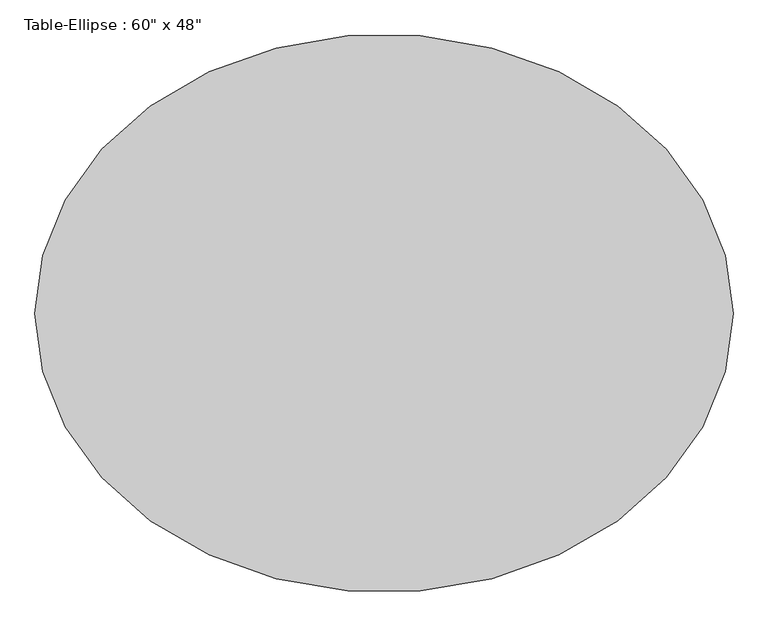
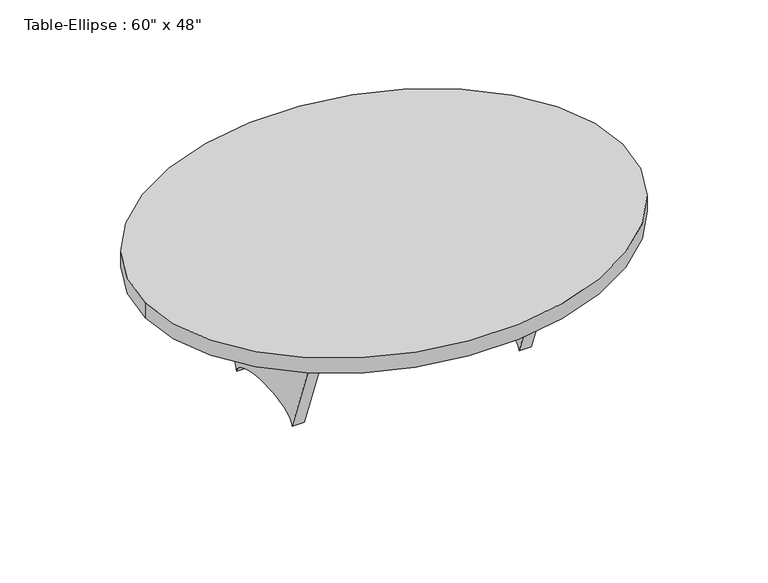
"""IFC4 building model written with IfcOpenShell, lengths in millimetres: furniture geometry."""

from ifc_helpers import new_model, si_unit, point, frame, origin, place, context, project, spatial, ellipse_curve, trimmed, source, transform, mapped, element, save
from ifc_brep_helpers import plane_surface, extruded_surface, advanced_brep


def furniture_c105135d(model_context):
    return source(origin(), model_context, "Body", "AdvancedBrep", [
        advanced_brep(
        [(-762.0, 0.0, 457.2), (762.0, 0.0, 457.2), (-762.0, 0.0, 406.4), (762.0, 0.0, 406.4)],
        [
            (0, 1, ellipse_curve(frame((0.0, 0.0, 457.2), z_axis=(0.0, 0.0, 1.0), x_axis=(1.0, 0.0, 0.0)), 762.0, 609.6)),
            (1, 0, ellipse_curve(frame((0.0, 0.0, 457.2), z_axis=(0.0, 0.0, 1.0), x_axis=(1.0, 0.0, 0.0)), 762.0, 609.6)),
            (2, 3, ellipse_curve(frame((0.0, 0.0, 406.4), z_axis=(0.0, 0.0, -1.0), x_axis=(1.0, 0.0, 0.0)), 762.0, 609.6)),
            (3, 2, ellipse_curve(frame((0.0, 0.0, 406.4), z_axis=(0.0, 0.0, -1.0), x_axis=(1.0, 0.0, 0.0)), 762.0, 609.6)),
            (0, 2),
            (3, 1),
        ],
        [
            plane_surface(frame((762.0, 0.0, 457.2), z_axis=(0.0, 0.0, 1.0), x_axis=(0.0, 1.0, 0.0))),
            plane_surface(frame((762.0, 0.0, 406.4), z_axis=(0.0, 0.0, -1.0), x_axis=(0.0, -1.0, 0.0))),
            extruded_surface(trimmed(ellipse_curve(frame((0.0, 0.0, 355.6), z_axis=(0.0, 0.0, 1.0), x_axis=(1.0, 0.0, 0.0)), 762.0, 609.6), [point((-762.0, 0.0, 355.6))], [point((762.0, 0.0, 355.6))], True, "CARTESIAN"), (0.0, 0.0, 50.799999999999955), 50.799999999999955),
            extruded_surface(trimmed(ellipse_curve(frame((0.0, 0.0, 355.6), z_axis=(0.0, 0.0, 1.0), x_axis=(1.0, 0.0, 0.0)), 762.0, 609.6), [point((762.0, 0.0, 355.6))], [point((-762.0, 0.0, 355.6))], True, "CARTESIAN"), (0.0, 0.0, 50.799999999999955), 50.799999999999955),
        ],
        [
            (0, [[1, 2]]),
            (1, [[3, 4]]),
            (2, [[-1, 5, -4, 6]]),
            (3, [[-2, -6, -3, -5]]),
        ],
    ),
        advanced_brep(
        [(-342.9, 304.8, 406.4), (-342.9, -304.8, 406.4), (-342.9, -152.4, 0.0), (-342.9, 152.4, 0.0), (-381.0, 304.8, 406.4), (-381.0, 152.4, 0.0), (-381.0, -152.4, 0.0), (-381.0, -304.8, 406.4)],
        [
            (0, 1),
            (1, 2),
            (2, 3, ellipse_curve(frame((-342.9, 0.0, 0.0), z_axis=(-1.0, 0.0, 0.0), x_axis=(0.0, 1.0, 0.0)), 152.4, 50.8)),
            (3, 0),
            (4, 5),
            (5, 6, ellipse_curve(frame((-381.0, 0.0, 0.0), z_axis=(1.0, 0.0, 0.0), x_axis=(0.0, 1.0, 0.0)), 152.4, 50.8)),
            (6, 7),
            (7, 4),
            (0, 4),
            (7, 1),
            (6, 2),
            (5, 3),
        ],
        [
            plane_surface(frame((-342.9, -304.8, 406.4), z_axis=(1.0, 0.0, 0.0), x_axis=(0.0, -1.0, 0.0))),
            plane_surface(frame((-381.0, -304.8, 406.4), z_axis=(-1.0, 0.0, 0.0), x_axis=(0.0, 1.0, 0.0))),
            plane_surface(frame((-342.9, 304.8, 406.4), z_axis=(0.0, 0.0, 1.0), x_axis=(-1.0, 0.0, 0.0))),
            plane_surface(frame((-342.9, -304.8, 406.4), z_axis=(0.0, -0.9363291775690403, -0.3511234415884029), x_axis=(-1.0, 0.0, 0.0))),
            extruded_surface(trimmed(ellipse_curve(frame((-419.1, 0.0, 0.0), z_axis=(-1.0, 0.0, 0.0), x_axis=(0.0, 1.0, 0.0)), 152.4, 50.8), [point((-419.1, -152.4, 0.0))], [point((-419.1, 152.4, 0.0))], True, "CARTESIAN"), (38.10000000000002, 0.0, 0.0), 38.10000000000002),
            plane_surface(frame((-342.9, 152.4, 0.0), z_axis=(0.0, 0.9363291775690458, -0.3511234415883884), x_axis=(-1.0, 0.0, 0.0))),
        ],
        [
            (0, [[1, 2, 3, 4]]),
            (1, [[5, 6, 7, 8]]),
            (2, [[-1, 9, -8, 10]]),
            (3, [[-2, -10, -7, 11]]),
            (4, [[-3, -11, -6, 12]]),
            (5, [[-4, -12, -5, -9]]),
        ],
    ),
        advanced_brep(
        [(381.0, 304.8, 406.4), (381.0, -304.8, 406.4), (381.0, -152.4, 0.0), (381.0, 152.4, 0.0), (342.9, 304.8, 406.4), (342.9, 152.4, 0.0), (342.9, -152.4, 0.0), (342.9, -304.8, 406.4)],
        [
            (0, 1),
            (1, 2),
            (2, 3, ellipse_curve(frame((381.0, 0.0, 0.0), z_axis=(-1.0, 0.0, 0.0), x_axis=(0.0, 1.0, 0.0)), 152.4, 50.8)),
            (3, 0),
            (4, 5),
            (5, 6, ellipse_curve(frame((342.9, 0.0, 0.0), z_axis=(1.0, 0.0, 0.0), x_axis=(0.0, 1.0, 0.0)), 152.4, 50.8)),
            (6, 7),
            (7, 4),
            (0, 4),
            (7, 1),
            (6, 2),
            (5, 3),
        ],
        [
            plane_surface(frame((381.0, -304.8, 406.4), z_axis=(1.0, 0.0, 0.0), x_axis=(0.0, -1.0, 0.0))),
            plane_surface(frame((342.9, -304.8, 406.4), z_axis=(-1.0, 0.0, 0.0), x_axis=(0.0, 1.0, 0.0))),
            plane_surface(frame((381.0, 304.8, 406.4), z_axis=(0.0, 0.0, 1.0), x_axis=(-1.0, 0.0, 0.0))),
            plane_surface(frame((381.0, -304.8, 406.4), z_axis=(0.0, -0.9363291775690407, -0.35112344158840214), x_axis=(-1.0, 0.0, 0.0))),
            extruded_surface(trimmed(ellipse_curve(frame((304.8, 0.0, 0.0), z_axis=(-1.0, 0.0, 0.0), x_axis=(0.0, 1.0, 0.0)), 152.4, 50.8), [point((304.8, -152.4, 0.0))], [point((304.8, 152.4, 0.0))], True, "CARTESIAN"), (38.099999999999966, 0.0, 0.0), 38.099999999999966),
            plane_surface(frame((381.0, 152.4, 0.0), z_axis=(0.0, 0.9363291775690474, -0.351123441588384), x_axis=(-1.0, 0.0, 0.0))),
        ],
        [
            (0, [[1, 2, 3, 4]]),
            (1, [[5, 6, 7, 8]]),
            (2, [[-1, 9, -8, 10]]),
            (3, [[-2, -10, -7, 11]]),
            (4, [[-3, -11, -6, 12]]),
            (5, [[-4, -12, -5, -9]]),
        ],
    ),
        advanced_brep(
        [(-342.9, 19.05, 406.4), (342.9, 19.05, 406.4), (342.9, 19.05, 270.9333333), (-342.9, 19.05, 270.9333333), (-342.9, -19.05, 406.4), (-342.9, -19.05, 270.9333333), (342.9, -19.05, 270.9333333), (342.9, -19.05, 406.4)],
        [
            (0, 1),
            (1, 2),
            (2, 3, ellipse_curve(frame((0.0, 19.05, 270.9333333), z_axis=(0.0, -1.0, 0.0), x_axis=(1.0, 0.0, 0.0)), 342.9, 101.6)),
            (3, 0),
            (4, 5),
            (5, 6, ellipse_curve(frame((0.0, -19.05, 270.9333333), z_axis=(0.0, 1.0, 0.0), x_axis=(1.0, 0.0, 0.0)), 342.9, 101.6)),
            (6, 7),
            (7, 4),
            (0, 4),
            (7, 1),
            (6, 2),
            (5, 3),
        ],
        [
            plane_surface(frame((-342.9, 19.05, 406.4), z_axis=(0.0, 1.0, 0.0), x_axis=(1.0, 0.0, 0.0))),
            plane_surface(frame((-342.9, -19.05, 406.4), z_axis=(0.0, -1.0, 0.0), x_axis=(-1.0, 0.0, 0.0))),
            plane_surface(frame((-342.9, 19.05, 406.4), z_axis=(0.0, 0.0, 1.0), x_axis=(0.0, -1.0, 0.0))),
            plane_surface(frame((342.9, 19.05, 406.4), z_axis=(1.0, 0.0, 0.0), x_axis=(0.0, -1.0, 0.0))),
            extruded_surface(trimmed(ellipse_curve(frame((0.0, -57.15, 270.9333333), z_axis=(0.0, -1.0, 0.0), x_axis=(1.0, 0.0, 0.0)), 342.9, 101.6), [point((342.9, -57.15, 270.9333333))], [point((-342.9, -57.15, 270.9333333))], True, "CARTESIAN"), (0.0, 38.099999999999994, 0.0), 38.099999999999994),
            plane_surface(frame((-342.9, 19.05, 270.9333333), z_axis=(-1.0, 0.0, 0.0), x_axis=(0.0, -1.0, 0.0))),
        ],
        [
            (0, [[1, 2, 3, 4]]),
            (1, [[5, 6, 7, 8]]),
            (2, [[-1, 9, -8, 10]]),
            (3, [[-2, -10, -7, 11]]),
            (4, [[-3, -11, -6, 12]]),
            (5, [[-4, -12, -5, -9]]),
        ],
    ),
    ])


if __name__ == "__main__":
    model = new_model("IFC4")
    model_context = context("Model", 3, world=origin())
    ifc_project = project(units=[si_unit("LENGTHUNIT", "METRE", prefix="MILLI")], contexts=[model_context])
    site = spatial("IfcSite", under=ifc_project)
    building = spatial("IfcBuilding", under=site)
    placement = place(None, origin())
    furniture_shape = furniture_c105135d(model_context)
    element("IfcFurniture", 1, ObjectType="Table-Ellipse : 60\" x 48\"", at=placement, inside=building, context=model_context, shape_type="MappedRepresentation", body=[
        mapped(furniture_shape, transform((0.0, 0.0, 0.0), x_axis=(1.0, 0.0, 0.0), y_axis=(0.0, 1.0, 0.0), z_axis=(0.0, 0.0, 1.0))),
    ])
    save(model, "model.ifc")

# Revit data of these elements
# Type "Table-Ellipse : 60\" x 48\""
#   Assembly Code = "E2020200"
#   Half Width = 2' - 0"
#   Half Length = 2' - 6"
#   Height = 1' - 6"
#   Length = 5' - 0"
#   Width = 4' - 0"
#   Base Material = Birch
#   Top Material = Birch
#   Default Elevation = 0
# Element 1 (IfcFurniture, "Table-Ellipse : 60\" x 48\"")
#   Materials on its faces: "Birch"
# Materials
#   "Birch": class "Wood", colour RGB 224 178 126, transparency 0, Description = "Betula Alleghaniensis", Cost = 0
